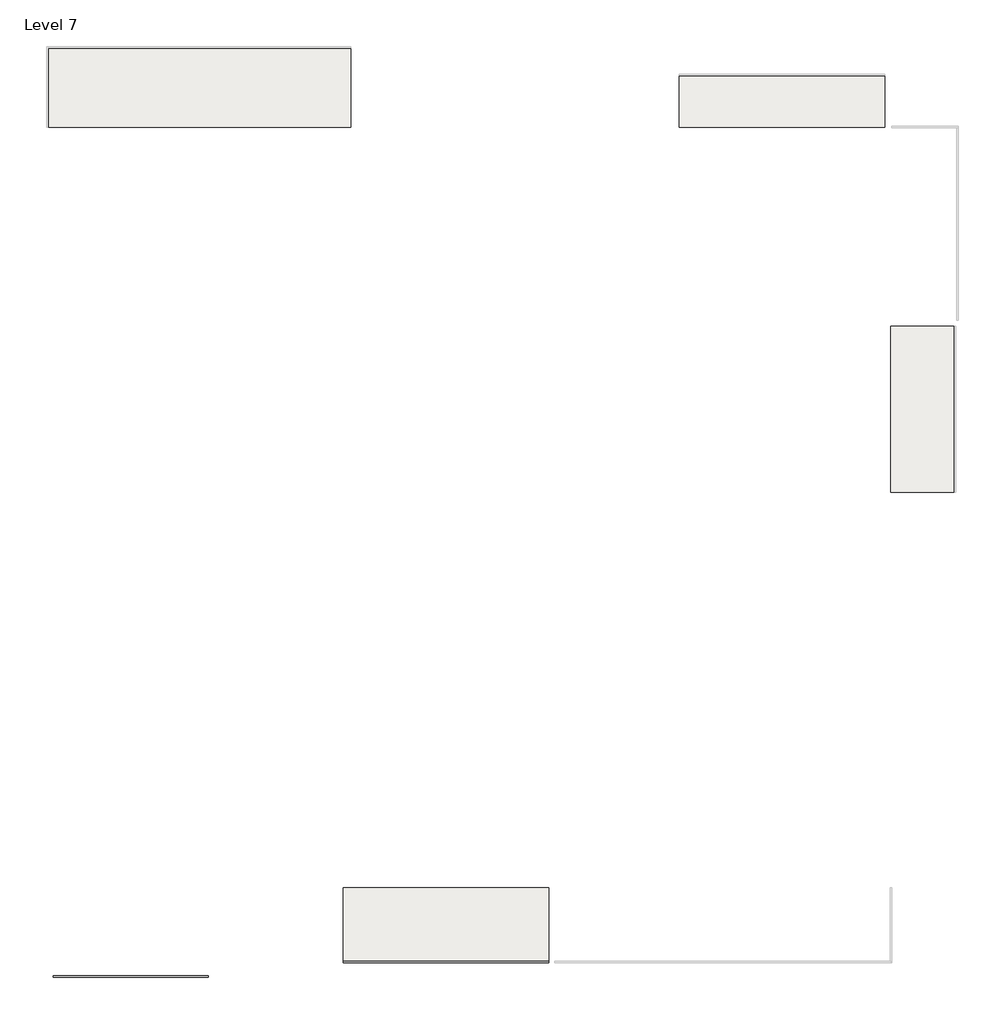
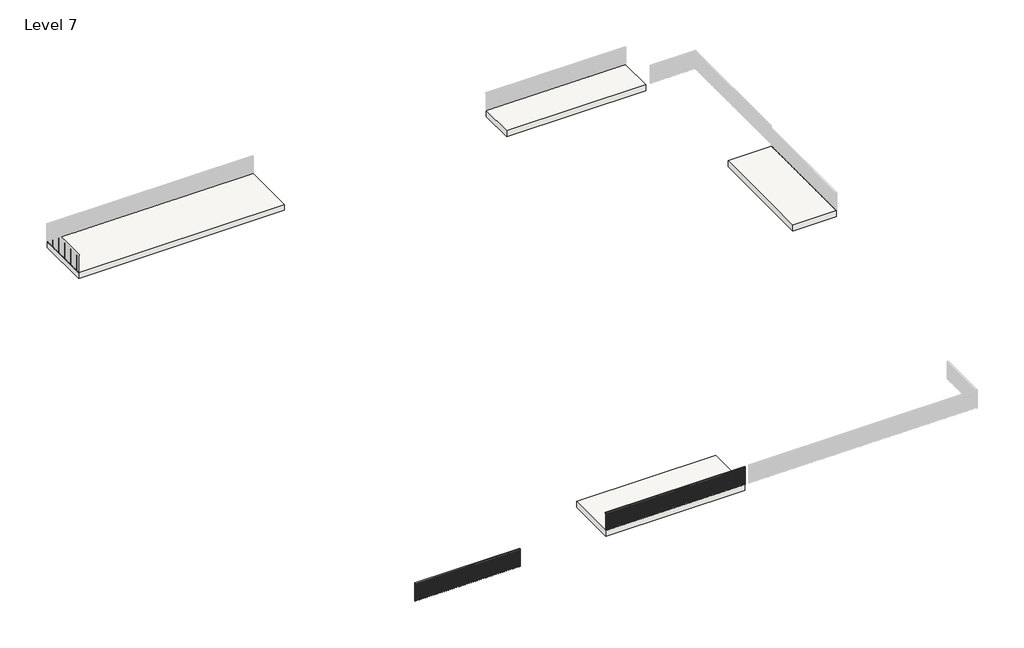
# One storey, part 1 of 5: 4 slabs, 2 railings.
"""IFC4 building model written with IfcOpenShell, lengths in millimetres."""

from ifc_helpers import new_model, si_unit, frame, origin, place, context, project, spatial, polyline, outline, extrude, element, save

model = new_model("IFC4")

# Units and contexts
model_context = context("Model", 3, world=origin())
ifc_project = project(units=[si_unit("LENGTHUNIT", "METRE", prefix="MILLI")], contexts=[model_context])

# Site, building, storey
site = spatial("IfcSite", under=ifc_project)
building = spatial("IfcBuilding", under=site)
storey = spatial("IfcBuildingStorey", under=building, Name="Level 7", Elevation=6400.8)

# Railings
placement = place(None, origin())
element("IfcRailing", 1, ObjectType="Handrail - Rectangular", at=placement, inside=storey, context=model_context, shape_type="SweptSolid", body=[
    extrude(outline(polyline([(-13630.2638778, -13399.9762475), (-13630.2638778, -13349.1762475), (-8499.4638778, -13349.1762475), (-8499.4638778, -13399.9762475), (-13630.2638778, -13399.9762475)])), frame((0.0, 0.0, 7264.4), z_axis=(0.0, 0.0, 1.0), x_axis=(1.0, 0.0, 0.0)), (0.0, 0.0, 1.0), 50.8),
    extrude(outline(polyline([(-8559.7888778, -13384.1012475), (-8559.7888778, -13365.0512475), (-8540.7388778, -13365.0512475), (-8540.7388778, -13384.1012475), (-8559.7888778, -13384.1012475)])), frame((0.0, 0.0, 6400.8), z_axis=(0.0, 0.0, 1.0), x_axis=(1.0, 0.0, 0.0)), (0.0, 0.0, 1.0), 863.6),
    extrude(outline(polyline([(-8661.3888778, -13384.1012475), (-8661.3888778, -13365.0512475), (-8642.3388778, -13365.0512475), (-8642.3388778, -13384.1012475), (-8661.3888778, -13384.1012475)])), frame((0.0, 0.0, 6400.8), z_axis=(0.0, 0.0, 1.0), x_axis=(1.0, 0.0, 0.0)), (0.0, 0.0, 1.0), 863.6),
    extrude(outline(polyline([(-8762.9888778, -13384.1012475), (-8762.9888778, -13365.0512475), (-8743.9388778, -13365.0512475), (-8743.9388778, -13384.1012475), (-8762.9888778, -13384.1012475)])), frame((0.0, 0.0, 6400.8), z_axis=(0.0, 0.0, 1.0), x_axis=(1.0, 0.0, 0.0)), (0.0, 0.0, 1.0), 863.6),
    extrude(outline(polyline([(-8864.5888778, -13384.1012475), (-8864.5888778, -13365.0512475), (-8845.5388778, -13365.0512475), (-8845.5388778, -13384.1012475), (-8864.5888778, -13384.1012475)])), frame((0.0, 0.0, 6400.8), z_axis=(0.0, 0.0, 1.0), x_axis=(1.0, 0.0, 0.0)), (0.0, 0.0, 1.0), 863.6),
    extrude(outline(polyline([(-8966.1888778, -13384.1012475), (-8966.1888778, -13365.0512475), (-8947.1388778, -13365.0512475), (-8947.1388778, -13384.1012475), (-8966.1888778, -13384.1012475)])), frame((0.0, 0.0, 6400.8), z_axis=(0.0, 0.0, 1.0), x_axis=(1.0, 0.0, 0.0)), (0.0, 0.0, 1.0), 863.6),
    extrude(outline(polyline([(-9067.7888778, -13384.1012475), (-9067.7888778, -13365.0512475), (-9048.7388778, -13365.0512475), (-9048.7388778, -13384.1012475), (-9067.7888778, -13384.1012475)])), frame((0.0, 0.0, 6400.8), z_axis=(0.0, 0.0, 1.0), x_axis=(1.0, 0.0, 0.0)), (0.0, 0.0, 1.0), 863.6),
    extrude(outline(polyline([(-9169.3888778, -13384.1012475), (-9169.3888778, -13365.0512475), (-9150.3388778, -13365.0512475), (-9150.3388778, -13384.1012475), (-9169.3888778, -13384.1012475)])), frame((0.0, 0.0, 6400.8), z_axis=(0.0, 0.0, 1.0), x_axis=(1.0, 0.0, 0.0)), (0.0, 0.0, 1.0), 863.6),
    extrude(outline(polyline([(-9270.9888778, -13384.1012475), (-9270.9888778, -13365.0512475), (-9251.9388778, -13365.0512475), (-9251.9388778, -13384.1012475), (-9270.9888778, -13384.1012475)])), frame((0.0, 0.0, 6400.8), z_axis=(0.0, 0.0, 1.0), x_axis=(1.0, 0.0, 0.0)), (0.0, 0.0, 1.0), 863.6),
    extrude(outline(polyline([(-9372.5888778, -13384.1012475), (-9372.5888778, -13365.0512475), (-9353.5388778, -13365.0512475), (-9353.5388778, -13384.1012475), (-9372.5888778, -13384.1012475)])), frame((0.0, 0.0, 6400.8), z_axis=(0.0, 0.0, 1.0), x_axis=(1.0, 0.0, 0.0)), (0.0, 0.0, 1.0), 863.6),
    extrude(outline(polyline([(-9474.1888778, -13384.1012475), (-9474.1888778, -13365.0512475), (-9455.1388778, -13365.0512475), (-9455.1388778, -13384.1012475), (-9474.1888778, -13384.1012475)])), frame((0.0, 0.0, 6400.8), z_axis=(0.0, 0.0, 1.0), x_axis=(1.0, 0.0, 0.0)), (0.0, 0.0, 1.0), 863.6),
    extrude(outline(polyline([(-9575.7888778, -13384.1012475), (-9575.7888778, -13365.0512475), (-9556.7388778, -13365.0512475), (-9556.7388778, -13384.1012475), (-9575.7888778, -13384.1012475)])), frame((0.0, 0.0, 6400.8), z_axis=(0.0, 0.0, 1.0), x_axis=(1.0, 0.0, 0.0)), (0.0, 0.0, 1.0), 863.6),
    extrude(outline(polyline([(-9677.3888778, -13384.1012475), (-9677.3888778, -13365.0512475), (-9658.3388778, -13365.0512475), (-9658.3388778, -13384.1012475), (-9677.3888778, -13384.1012475)])), frame((0.0, 0.0, 6400.8), z_axis=(0.0, 0.0, 1.0), x_axis=(1.0, 0.0, 0.0)), (0.0, 0.0, 1.0), 863.6),
    extrude(outline(polyline([(-9778.9888778, -13384.1012475), (-9778.9888778, -13365.0512475), (-9759.9388778, -13365.0512475), (-9759.9388778, -13384.1012475), (-9778.9888778, -13384.1012475)])), frame((0.0, 0.0, 6400.8), z_axis=(0.0, 0.0, 1.0), x_axis=(1.0, 0.0, 0.0)), (0.0, 0.0, 1.0), 863.6),
    extrude(outline(polyline([(-9880.5888778, -13384.1012475), (-9880.5888778, -13365.0512475), (-9861.5388778, -13365.0512475), (-9861.5388778, -13384.1012475), (-9880.5888778, -13384.1012475)])), frame((0.0, 0.0, 6400.8), z_axis=(0.0, 0.0, 1.0), x_axis=(1.0, 0.0, 0.0)), (0.0, 0.0, 1.0), 863.6),
    extrude(outline(polyline([(-9982.1888778, -13384.1012475), (-9982.1888778, -13365.0512475), (-9963.1388778, -13365.0512475), (-9963.1388778, -13384.1012475), (-9982.1888778, -13384.1012475)])), frame((0.0, 0.0, 6400.8), z_axis=(0.0, 0.0, 1.0), x_axis=(1.0, 0.0, 0.0)), (0.0, 0.0, 1.0), 863.6),
    extrude(outline(polyline([(-10083.7888778, -13384.1012475), (-10083.7888778, -13365.0512475), (-10064.7388778, -13365.0512475), (-10064.7388778, -13384.1012475), (-10083.7888778, -13384.1012475)])), frame((0.0, 0.0, 6400.8), z_axis=(0.0, 0.0, 1.0), x_axis=(1.0, 0.0, 0.0)), (0.0, 0.0, 1.0), 863.6),
    extrude(outline(polyline([(-10185.3888778, -13384.1012475), (-10185.3888778, -13365.0512475), (-10166.3388778, -13365.0512475), (-10166.3388778, -13384.1012475), (-10185.3888778, -13384.1012475)])), frame((0.0, 0.0, 6400.8), z_axis=(0.0, 0.0, 1.0), x_axis=(1.0, 0.0, 0.0)), (0.0, 0.0, 1.0), 863.6),
    extrude(outline(polyline([(-10286.9888778, -13384.1012475), (-10286.9888778, -13365.0512475), (-10267.9388778, -13365.0512475), (-10267.9388778, -13384.1012475), (-10286.9888778, -13384.1012475)])), frame((0.0, 0.0, 6400.8), z_axis=(0.0, 0.0, 1.0), x_axis=(1.0, 0.0, 0.0)), (0.0, 0.0, 1.0), 863.6),
    extrude(outline(polyline([(-10388.5888778, -13384.1012475), (-10388.5888778, -13365.0512475), (-10369.5388778, -13365.0512475), (-10369.5388778, -13384.1012475), (-10388.5888778, -13384.1012475)])), frame((0.0, 0.0, 6400.8), z_axis=(0.0, 0.0, 1.0), x_axis=(1.0, 0.0, 0.0)), (0.0, 0.0, 1.0), 863.6),
    extrude(outline(polyline([(-10490.1888778, -13384.1012475), (-10490.1888778, -13365.0512475), (-10471.1388778, -13365.0512475), (-10471.1388778, -13384.1012475), (-10490.1888778, -13384.1012475)])), frame((0.0, 0.0, 6400.8), z_axis=(0.0, 0.0, 1.0), x_axis=(1.0, 0.0, 0.0)), (0.0, 0.0, 1.0), 863.6),
    extrude(outline(polyline([(-10591.7888778, -13384.1012475), (-10591.7888778, -13365.0512475), (-10572.7388778, -13365.0512475), (-10572.7388778, -13384.1012475), (-10591.7888778, -13384.1012475)])), frame((0.0, 0.0, 6400.8), z_axis=(0.0, 0.0, 1.0), x_axis=(1.0, 0.0, 0.0)), (0.0, 0.0, 1.0), 863.6),
    extrude(outline(polyline([(-10693.3888778, -13384.1012475), (-10693.3888778, -13365.0512475), (-10674.3388778, -13365.0512475), (-10674.3388778, -13384.1012475), (-10693.3888778, -13384.1012475)])), frame((0.0, 0.0, 6400.8), z_axis=(0.0, 0.0, 1.0), x_axis=(1.0, 0.0, 0.0)), (0.0, 0.0, 1.0), 863.6),
    extrude(outline(polyline([(-10794.9888778, -13384.1012475), (-10794.9888778, -13365.0512475), (-10775.9388778, -13365.0512475), (-10775.9388778, -13384.1012475), (-10794.9888778, -13384.1012475)])), frame((0.0, 0.0, 6400.8), z_axis=(0.0, 0.0, 1.0), x_axis=(1.0, 0.0, 0.0)), (0.0, 0.0, 1.0), 863.6),
    extrude(outline(polyline([(-10896.5888778, -13384.1012475), (-10896.5888778, -13365.0512475), (-10877.5388778, -13365.0512475), (-10877.5388778, -13384.1012475), (-10896.5888778, -13384.1012475)])), frame((0.0, 0.0, 6400.8), z_axis=(0.0, 0.0, 1.0), x_axis=(1.0, 0.0, 0.0)), (0.0, 0.0, 1.0), 863.6),
    extrude(outline(polyline([(-10998.1888778, -13384.1012475), (-10998.1888778, -13365.0512475), (-10979.1388778, -13365.0512475), (-10979.1388778, -13384.1012475), (-10998.1888778, -13384.1012475)])), frame((0.0, 0.0, 6400.8), z_axis=(0.0, 0.0, 1.0), x_axis=(1.0, 0.0, 0.0)), (0.0, 0.0, 1.0), 863.6),
    extrude(outline(polyline([(-11099.7888778, -13384.1012475), (-11099.7888778, -13365.0512475), (-11080.7388778, -13365.0512475), (-11080.7388778, -13384.1012475), (-11099.7888778, -13384.1012475)])), frame((0.0, 0.0, 6400.8), z_axis=(0.0, 0.0, 1.0), x_axis=(1.0, 0.0, 0.0)), (0.0, 0.0, 1.0), 863.6),
    extrude(outline(polyline([(-11201.3888778, -13384.1012475), (-11201.3888778, -13365.0512475), (-11182.3388778, -13365.0512475), (-11182.3388778, -13384.1012475), (-11201.3888778, -13384.1012475)])), frame((0.0, 0.0, 6400.8), z_axis=(0.0, 0.0, 1.0), x_axis=(1.0, 0.0, 0.0)), (0.0, 0.0, 1.0), 863.6),
    extrude(outline(polyline([(-11302.9888778, -13384.1012475), (-11302.9888778, -13365.0512475), (-11283.9388778, -13365.0512475), (-11283.9388778, -13384.1012475), (-11302.9888778, -13384.1012475)])), frame((0.0, 0.0, 6400.8), z_axis=(0.0, 0.0, 1.0), x_axis=(1.0, 0.0, 0.0)), (0.0, 0.0, 1.0), 863.6),
    extrude(outline(polyline([(-11404.5888778, -13384.1012475), (-11404.5888778, -13365.0512475), (-11385.5388778, -13365.0512475), (-11385.5388778, -13384.1012475), (-11404.5888778, -13384.1012475)])), frame((0.0, 0.0, 6400.8), z_axis=(0.0, 0.0, 1.0), x_axis=(1.0, 0.0, 0.0)), (0.0, 0.0, 1.0), 863.6),
    extrude(outline(polyline([(-11506.1888778, -13384.1012475), (-11506.1888778, -13365.0512475), (-11487.1388778, -13365.0512475), (-11487.1388778, -13384.1012475), (-11506.1888778, -13384.1012475)])), frame((0.0, 0.0, 6400.8), z_axis=(0.0, 0.0, 1.0), x_axis=(1.0, 0.0, 0.0)), (0.0, 0.0, 1.0), 863.6),
    extrude(outline(polyline([(-11607.7888778, -13384.1012475), (-11607.7888778, -13365.0512475), (-11588.7388778, -13365.0512475), (-11588.7388778, -13384.1012475), (-11607.7888778, -13384.1012475)])), frame((0.0, 0.0, 6400.8), z_axis=(0.0, 0.0, 1.0), x_axis=(1.0, 0.0, 0.0)), (0.0, 0.0, 1.0), 863.6),
    extrude(outline(polyline([(-11709.3888778, -13384.1012475), (-11709.3888778, -13365.0512475), (-11690.3388778, -13365.0512475), (-11690.3388778, -13384.1012475), (-11709.3888778, -13384.1012475)])), frame((0.0, 0.0, 6400.8), z_axis=(0.0, 0.0, 1.0), x_axis=(1.0, 0.0, 0.0)), (0.0, 0.0, 1.0), 863.6),
    extrude(outline(polyline([(-11810.9888778, -13384.1012475), (-11810.9888778, -13365.0512475), (-11791.9388778, -13365.0512475), (-11791.9388778, -13384.1012475), (-11810.9888778, -13384.1012475)])), frame((0.0, 0.0, 6400.8), z_axis=(0.0, 0.0, 1.0), x_axis=(1.0, 0.0, 0.0)), (0.0, 0.0, 1.0), 863.6),
    extrude(outline(polyline([(-11912.5888778, -13384.1012475), (-11912.5888778, -13365.0512475), (-11893.5388778, -13365.0512475), (-11893.5388778, -13384.1012475), (-11912.5888778, -13384.1012475)])), frame((0.0, 0.0, 6400.8), z_axis=(0.0, 0.0, 1.0), x_axis=(1.0, 0.0, 0.0)), (0.0, 0.0, 1.0), 863.6),
    extrude(outline(polyline([(-12014.1888778, -13384.1012475), (-12014.1888778, -13365.0512475), (-11995.1388778, -13365.0512475), (-11995.1388778, -13384.1012475), (-12014.1888778, -13384.1012475)])), frame((0.0, 0.0, 6400.8), z_axis=(0.0, 0.0, 1.0), x_axis=(1.0, 0.0, 0.0)), (0.0, 0.0, 1.0), 863.6),
    extrude(outline(polyline([(-12115.7888778, -13384.1012475), (-12115.7888778, -13365.0512475), (-12096.7388778, -13365.0512475), (-12096.7388778, -13384.1012475), (-12115.7888778, -13384.1012475)])), frame((0.0, 0.0, 6400.8), z_axis=(0.0, 0.0, 1.0), x_axis=(1.0, 0.0, 0.0)), (0.0, 0.0, 1.0), 863.6),
    extrude(outline(polyline([(-12217.3888778, -13384.1012475), (-12217.3888778, -13365.0512475), (-12198.3388778, -13365.0512475), (-12198.3388778, -13384.1012475), (-12217.3888778, -13384.1012475)])), frame((0.0, 0.0, 6400.8), z_axis=(0.0, 0.0, 1.0), x_axis=(1.0, 0.0, 0.0)), (0.0, 0.0, 1.0), 863.6),
    extrude(outline(polyline([(-12318.9888778, -13384.1012475), (-12318.9888778, -13365.0512475), (-12299.9388778, -13365.0512475), (-12299.9388778, -13384.1012475), (-12318.9888778, -13384.1012475)])), frame((0.0, 0.0, 6400.8), z_axis=(0.0, 0.0, 1.0), x_axis=(1.0, 0.0, 0.0)), (0.0, 0.0, 1.0), 863.6),
    extrude(outline(polyline([(-12420.5888778, -13384.1012475), (-12420.5888778, -13365.0512475), (-12401.5388778, -13365.0512475), (-12401.5388778, -13384.1012475), (-12420.5888778, -13384.1012475)])), frame((0.0, 0.0, 6400.8), z_axis=(0.0, 0.0, 1.0), x_axis=(1.0, 0.0, 0.0)), (0.0, 0.0, 1.0), 863.6),
    extrude(outline(polyline([(-12522.1888778, -13384.1012475), (-12522.1888778, -13365.0512475), (-12503.1388778, -13365.0512475), (-12503.1388778, -13384.1012475), (-12522.1888778, -13384.1012475)])), frame((0.0, 0.0, 6400.8), z_axis=(0.0, 0.0, 1.0), x_axis=(1.0, 0.0, 0.0)), (0.0, 0.0, 1.0), 863.6),
    extrude(outline(polyline([(-12623.7888778, -13384.1012475), (-12623.7888778, -13365.0512475), (-12604.7388778, -13365.0512475), (-12604.7388778, -13384.1012475), (-12623.7888778, -13384.1012475)])), frame((0.0, 0.0, 6400.8), z_axis=(0.0, 0.0, 1.0), x_axis=(1.0, 0.0, 0.0)), (0.0, 0.0, 1.0), 863.6),
    extrude(outline(polyline([(-12725.3888778, -13384.1012475), (-12725.3888778, -13365.0512475), (-12706.3388778, -13365.0512475), (-12706.3388778, -13384.1012475), (-12725.3888778, -13384.1012475)])), frame((0.0, 0.0, 6400.8), z_axis=(0.0, 0.0, 1.0), x_axis=(1.0, 0.0, 0.0)), (0.0, 0.0, 1.0), 863.6),
    extrude(outline(polyline([(-12826.9888778, -13384.1012475), (-12826.9888778, -13365.0512475), (-12807.9388778, -13365.0512475), (-12807.9388778, -13384.1012475), (-12826.9888778, -13384.1012475)])), frame((0.0, 0.0, 6400.8), z_axis=(0.0, 0.0, 1.0), x_axis=(1.0, 0.0, 0.0)), (0.0, 0.0, 1.0), 863.6),
    extrude(outline(polyline([(-12928.5888778, -13384.1012475), (-12928.5888778, -13365.0512475), (-12909.5388778, -13365.0512475), (-12909.5388778, -13384.1012475), (-12928.5888778, -13384.1012475)])), frame((0.0, 0.0, 6400.8), z_axis=(0.0, 0.0, 1.0), x_axis=(1.0, 0.0, 0.0)), (0.0, 0.0, 1.0), 863.6),
    extrude(outline(polyline([(-13030.1888778, -13384.1012475), (-13030.1888778, -13365.0512475), (-13011.1388778, -13365.0512475), (-13011.1388778, -13384.1012475), (-13030.1888778, -13384.1012475)])), frame((0.0, 0.0, 6400.8), z_axis=(0.0, 0.0, 1.0), x_axis=(1.0, 0.0, 0.0)), (0.0, 0.0, 1.0), 863.6),
    extrude(outline(polyline([(-13131.7888778, -13384.1012475), (-13131.7888778, -13365.0512475), (-13112.7388778, -13365.0512475), (-13112.7388778, -13384.1012475), (-13131.7888778, -13384.1012475)])), frame((0.0, 0.0, 6400.8), z_axis=(0.0, 0.0, 1.0), x_axis=(1.0, 0.0, 0.0)), (0.0, 0.0, 1.0), 863.6),
    extrude(outline(polyline([(-13233.3888778, -13384.1012475), (-13233.3888778, -13365.0512475), (-13214.3388778, -13365.0512475), (-13214.3388778, -13384.1012475), (-13233.3888778, -13384.1012475)])), frame((0.0, 0.0, 6400.8), z_axis=(0.0, 0.0, 1.0), x_axis=(1.0, 0.0, 0.0)), (0.0, 0.0, 1.0), 863.6),
    extrude(outline(polyline([(-13334.9888778, -13384.1012475), (-13334.9888778, -13365.0512475), (-13315.9388778, -13365.0512475), (-13315.9388778, -13384.1012475), (-13334.9888778, -13384.1012475)])), frame((0.0, 0.0, 6400.8), z_axis=(0.0, 0.0, 1.0), x_axis=(1.0, 0.0, 0.0)), (0.0, 0.0, 1.0), 863.6),
    extrude(outline(polyline([(-13436.5888778, -13384.1012475), (-13436.5888778, -13365.0512475), (-13417.5388778, -13365.0512475), (-13417.5388778, -13384.1012475), (-13436.5888778, -13384.1012475)])), frame((0.0, 0.0, 6400.8), z_axis=(0.0, 0.0, 1.0), x_axis=(1.0, 0.0, 0.0)), (0.0, 0.0, 1.0), 863.6),
    extrude(outline(polyline([(-13538.1888778, -13384.1012475), (-13538.1888778, -13365.0512475), (-13519.1388778, -13365.0512475), (-13519.1388778, -13384.1012475), (-13538.1888778, -13384.1012475)])), frame((0.0, 0.0, 6400.8), z_axis=(0.0, 0.0, 1.0), x_axis=(1.0, 0.0, 0.0)), (0.0, 0.0, 1.0), 863.6),
    extrude(outline(polyline([(-8518.5138778, -13384.1012475), (-8518.5138778, -13365.0512475), (-8499.4638778, -13365.0512475), (-8499.4638778, -13384.1012475), (-8518.5138778, -13384.1012475)])), frame((0.0, 0.0, 6400.8), z_axis=(0.0, 0.0, 1.0), x_axis=(1.0, 0.0, 0.0)), (0.0, 0.0, 1.0), 863.6),
    extrude(outline(polyline([(-13630.2638778, -13384.1012475), (-13630.2638778, -13365.0512475), (-13611.2138778, -13365.0512475), (-13611.2138778, -13384.1012475), (-13630.2638778, -13384.1012475)])), frame((0.0, 0.0, 6400.8), z_axis=(0.0, 0.0, 1.0), x_axis=(1.0, 0.0, 0.0)), (0.0, 0.0, 1.0), 863.6),
])
element("IfcRailing", 2, ObjectType="Handrail - Rectangular", at=placement, inside=storey, context=model_context, shape_type="SweptSolid", body=[
    extrude(outline(polyline([(-4029.0638778, -12911.7749501), (-4029.0638778, -12860.9749501), (2778.1361222, -12860.9749501), (2778.1361222, -12911.7749501), (-4029.0638778, -12911.7749501)])), frame((0.0, 0.0, 7264.4), z_axis=(0.0, 0.0, 1.0), x_axis=(1.0, 0.0, 0.0)), (0.0, 0.0, 1.0), 50.8),
    extrude(outline(polyline([(2667.0111222, -12895.8999501), (2667.0111222, -12876.8499501), (2686.0611222, -12876.8499501), (2686.0611222, -12895.8999501), (2667.0111222, -12895.8999501)])), frame((0.0, 0.0, 6400.8), z_axis=(0.0, 0.0, 1.0), x_axis=(1.0, 0.0, 0.0)), (0.0, 0.0, 1.0), 863.6),
    extrude(outline(polyline([(2565.4111222, -12895.8999501), (2565.4111222, -12876.8499501), (2584.4611222, -12876.8499501), (2584.4611222, -12895.8999501), (2565.4111222, -12895.8999501)])), frame((0.0, 0.0, 6400.8), z_axis=(0.0, 0.0, 1.0), x_axis=(1.0, 0.0, 0.0)), (0.0, 0.0, 1.0), 863.6),
    extrude(outline(polyline([(2463.8111222, -12895.8999501), (2463.8111222, -12876.8499501), (2482.8611222, -12876.8499501), (2482.8611222, -12895.8999501), (2463.8111222, -12895.8999501)])), frame((0.0, 0.0, 6400.8), z_axis=(0.0, 0.0, 1.0), x_axis=(1.0, 0.0, 0.0)), (0.0, 0.0, 1.0), 863.6),
    extrude(outline(polyline([(2362.2111222, -12895.8999501), (2362.2111222, -12876.8499501), (2381.2611222, -12876.8499501), (2381.2611222, -12895.8999501), (2362.2111222, -12895.8999501)])), frame((0.0, 0.0, 6400.8), z_axis=(0.0, 0.0, 1.0), x_axis=(1.0, 0.0, 0.0)), (0.0, 0.0, 1.0), 863.6),
    extrude(outline(polyline([(2260.6111222, -12895.8999501), (2260.6111222, -12876.8499501), (2279.6611222, -12876.8499501), (2279.6611222, -12895.8999501), (2260.6111222, -12895.8999501)])), frame((0.0, 0.0, 6400.8), z_axis=(0.0, 0.0, 1.0), x_axis=(1.0, 0.0, 0.0)), (0.0, 0.0, 1.0), 863.6),
    extrude(outline(polyline([(2159.0111222, -12895.8999501), (2159.0111222, -12876.8499501), (2178.0611222, -12876.8499501), (2178.0611222, -12895.8999501), (2159.0111222, -12895.8999501)])), frame((0.0, 0.0, 6400.8), z_axis=(0.0, 0.0, 1.0), x_axis=(1.0, 0.0, 0.0)), (0.0, 0.0, 1.0), 863.6),
    extrude(outline(polyline([(2057.4111222, -12895.8999501), (2057.4111222, -12876.8499501), (2076.4611222, -12876.8499501), (2076.4611222, -12895.8999501), (2057.4111222, -12895.8999501)])), frame((0.0, 0.0, 6400.8), z_axis=(0.0, 0.0, 1.0), x_axis=(1.0, 0.0, 0.0)), (0.0, 0.0, 1.0), 863.6),
    extrude(outline(polyline([(1955.8111222, -12895.8999501), (1955.8111222, -12876.8499501), (1974.8611222, -12876.8499501), (1974.8611222, -12895.8999501), (1955.8111222, -12895.8999501)])), frame((0.0, 0.0, 6400.8), z_axis=(0.0, 0.0, 1.0), x_axis=(1.0, 0.0, 0.0)), (0.0, 0.0, 1.0), 863.6),
    extrude(outline(polyline([(1854.2111222, -12895.8999501), (1854.2111222, -12876.8499501), (1873.2611222, -12876.8499501), (1873.2611222, -12895.8999501), (1854.2111222, -12895.8999501)])), frame((0.0, 0.0, 6400.8), z_axis=(0.0, 0.0, 1.0), x_axis=(1.0, 0.0, 0.0)), (0.0, 0.0, 1.0), 863.6),
    extrude(outline(polyline([(1752.6111222, -12895.8999501), (1752.6111222, -12876.8499501), (1771.6611222, -12876.8499501), (1771.6611222, -12895.8999501), (1752.6111222, -12895.8999501)])), frame((0.0, 0.0, 6400.8), z_axis=(0.0, 0.0, 1.0), x_axis=(1.0, 0.0, 0.0)), (0.0, 0.0, 1.0), 863.6),
    extrude(outline(polyline([(1651.0111222, -12895.8999501), (1651.0111222, -12876.8499501), (1670.0611222, -12876.8499501), (1670.0611222, -12895.8999501), (1651.0111222, -12895.8999501)])), frame((0.0, 0.0, 6400.8), z_axis=(0.0, 0.0, 1.0), x_axis=(1.0, 0.0, 0.0)), (0.0, 0.0, 1.0), 863.6),
    extrude(outline(polyline([(1549.4111222, -12895.8999501), (1549.4111222, -12876.8499501), (1568.4611222, -12876.8499501), (1568.4611222, -12895.8999501), (1549.4111222, -12895.8999501)])), frame((0.0, 0.0, 6400.8), z_axis=(0.0, 0.0, 1.0), x_axis=(1.0, 0.0, 0.0)), (0.0, 0.0, 1.0), 863.6),
    extrude(outline(polyline([(1447.8111222, -12895.8999501), (1447.8111222, -12876.8499501), (1466.8611222, -12876.8499501), (1466.8611222, -12895.8999501), (1447.8111222, -12895.8999501)])), frame((0.0, 0.0, 6400.8), z_axis=(0.0, 0.0, 1.0), x_axis=(1.0, 0.0, 0.0)), (0.0, 0.0, 1.0), 863.6),
    extrude(outline(polyline([(1346.2111222, -12895.8999501), (1346.2111222, -12876.8499501), (1365.2611222, -12876.8499501), (1365.2611222, -12895.8999501), (1346.2111222, -12895.8999501)])), frame((0.0, 0.0, 6400.8), z_axis=(0.0, 0.0, 1.0), x_axis=(1.0, 0.0, 0.0)), (0.0, 0.0, 1.0), 863.6),
    extrude(outline(polyline([(1244.6111222, -12895.8999501), (1244.6111222, -12876.8499501), (1263.6611222, -12876.8499501), (1263.6611222, -12895.8999501), (1244.6111222, -12895.8999501)])), frame((0.0, 0.0, 6400.8), z_axis=(0.0, 0.0, 1.0), x_axis=(1.0, 0.0, 0.0)), (0.0, 0.0, 1.0), 863.6),
    extrude(outline(polyline([(1143.0111222, -12895.8999501), (1143.0111222, -12876.8499501), (1162.0611222, -12876.8499501), (1162.0611222, -12895.8999501), (1143.0111222, -12895.8999501)])), frame((0.0, 0.0, 6400.8), z_axis=(0.0, 0.0, 1.0), x_axis=(1.0, 0.0, 0.0)), (0.0, 0.0, 1.0), 863.6),
    extrude(outline(polyline([(1041.4111222, -12895.8999501), (1041.4111222, -12876.8499501), (1060.4611222, -12876.8499501), (1060.4611222, -12895.8999501), (1041.4111222, -12895.8999501)])), frame((0.0, 0.0, 6400.8), z_axis=(0.0, 0.0, 1.0), x_axis=(1.0, 0.0, 0.0)), (0.0, 0.0, 1.0), 863.6),
    extrude(outline(polyline([(939.8111222, -12895.8999501), (939.8111222, -12876.8499501), (958.8611222, -12876.8499501), (958.8611222, -12895.8999501), (939.8111222, -12895.8999501)])), frame((0.0, 0.0, 6400.8), z_axis=(0.0, 0.0, 1.0), x_axis=(1.0, 0.0, 0.0)), (0.0, 0.0, 1.0), 863.6),
    extrude(outline(polyline([(838.2111222, -12895.8999501), (838.2111222, -12876.8499501), (857.2611222, -12876.8499501), (857.2611222, -12895.8999501), (838.2111222, -12895.8999501)])), frame((0.0, 0.0, 6400.8), z_axis=(0.0, 0.0, 1.0), x_axis=(1.0, 0.0, 0.0)), (0.0, 0.0, 1.0), 863.6),
    extrude(outline(polyline([(736.6111222, -12895.8999501), (736.6111222, -12876.8499501), (755.6611222, -12876.8499501), (755.6611222, -12895.8999501), (736.6111222, -12895.8999501)])), frame((0.0, 0.0, 6400.8), z_axis=(0.0, 0.0, 1.0), x_axis=(1.0, 0.0, 0.0)), (0.0, 0.0, 1.0), 863.6),
    extrude(outline(polyline([(635.0111222, -12895.8999501), (635.0111222, -12876.8499501), (654.0611222, -12876.8499501), (654.0611222, -12895.8999501), (635.0111222, -12895.8999501)])), frame((0.0, 0.0, 6400.8), z_axis=(0.0, 0.0, 1.0), x_axis=(1.0, 0.0, 0.0)), (0.0, 0.0, 1.0), 863.6),
    extrude(outline(polyline([(533.4111222, -12895.8999501), (533.4111222, -12876.8499501), (552.4611222, -12876.8499501), (552.4611222, -12895.8999501), (533.4111222, -12895.8999501)])), frame((0.0, 0.0, 6400.8), z_axis=(0.0, 0.0, 1.0), x_axis=(1.0, 0.0, 0.0)), (0.0, 0.0, 1.0), 863.6),
    extrude(outline(polyline([(431.8111222, -12895.8999501), (431.8111222, -12876.8499501), (450.8611222, -12876.8499501), (450.8611222, -12895.8999501), (431.8111222, -12895.8999501)])), frame((0.0, 0.0, 6400.8), z_axis=(0.0, 0.0, 1.0), x_axis=(1.0, 0.0, 0.0)), (0.0, 0.0, 1.0), 863.6),
    extrude(outline(polyline([(330.2111222, -12895.8999501), (330.2111222, -12876.8499501), (349.2611222, -12876.8499501), (349.2611222, -12895.8999501), (330.2111222, -12895.8999501)])), frame((0.0, 0.0, 6400.8), z_axis=(0.0, 0.0, 1.0), x_axis=(1.0, 0.0, 0.0)), (0.0, 0.0, 1.0), 863.6),
    extrude(outline(polyline([(228.6111222, -12895.8999501), (228.6111222, -12876.8499501), (247.6611222, -12876.8499501), (247.6611222, -12895.8999501), (228.6111222, -12895.8999501)])), frame((0.0, 0.0, 6400.8), z_axis=(0.0, 0.0, 1.0), x_axis=(1.0, 0.0, 0.0)), (0.0, 0.0, 1.0), 863.6),
    extrude(outline(polyline([(127.0111222, -12895.8999501), (127.0111222, -12876.8499501), (146.0611222, -12876.8499501), (146.0611222, -12895.8999501), (127.0111222, -12895.8999501)])), frame((0.0, 0.0, 6400.8), z_axis=(0.0, 0.0, 1.0), x_axis=(1.0, 0.0, 0.0)), (0.0, 0.0, 1.0), 863.6),
    extrude(outline(polyline([(25.4111222, -12895.8999501), (25.4111222, -12876.8499501), (44.4611222, -12876.8499501), (44.4611222, -12895.8999501), (25.4111222, -12895.8999501)])), frame((0.0, 0.0, 6400.8), z_axis=(0.0, 0.0, 1.0), x_axis=(1.0, 0.0, 0.0)), (0.0, 0.0, 1.0), 863.6),
    extrude(outline(polyline([(-76.1888778, -12895.8999501), (-76.1888778, -12876.8499501), (-57.1388778, -12876.8499501), (-57.1388778, -12895.8999501), (-76.1888778, -12895.8999501)])), frame((0.0, 0.0, 6400.8), z_axis=(0.0, 0.0, 1.0), x_axis=(1.0, 0.0, 0.0)), (0.0, 0.0, 1.0), 863.6),
    extrude(outline(polyline([(-177.7888778, -12895.8999501), (-177.7888778, -12876.8499501), (-158.7388778, -12876.8499501), (-158.7388778, -12895.8999501), (-177.7888778, -12895.8999501)])), frame((0.0, 0.0, 6400.8), z_axis=(0.0, 0.0, 1.0), x_axis=(1.0, 0.0, 0.0)), (0.0, 0.0, 1.0), 863.6),
    extrude(outline(polyline([(-279.3888778, -12895.8999501), (-279.3888778, -12876.8499501), (-260.3388778, -12876.8499501), (-260.3388778, -12895.8999501), (-279.3888778, -12895.8999501)])), frame((0.0, 0.0, 6400.8), z_axis=(0.0, 0.0, 1.0), x_axis=(1.0, 0.0, 0.0)), (0.0, 0.0, 1.0), 863.6),
    extrude(outline(polyline([(-380.9888778, -12895.8999501), (-380.9888778, -12876.8499501), (-361.9388778, -12876.8499501), (-361.9388778, -12895.8999501), (-380.9888778, -12895.8999501)])), frame((0.0, 0.0, 6400.8), z_axis=(0.0, 0.0, 1.0), x_axis=(1.0, 0.0, 0.0)), (0.0, 0.0, 1.0), 863.6),
    extrude(outline(polyline([(-482.5888778, -12895.8999501), (-482.5888778, -12876.8499501), (-463.5388778, -12876.8499501), (-463.5388778, -12895.8999501), (-482.5888778, -12895.8999501)])), frame((0.0, 0.0, 6400.8), z_axis=(0.0, 0.0, 1.0), x_axis=(1.0, 0.0, 0.0)), (0.0, 0.0, 1.0), 863.6),
    extrude(outline(polyline([(-584.1888778, -12895.8999501), (-584.1888778, -12876.8499501), (-565.1388778, -12876.8499501), (-565.1388778, -12895.8999501), (-584.1888778, -12895.8999501)])), frame((0.0, 0.0, 6400.8), z_axis=(0.0, 0.0, 1.0), x_axis=(1.0, 0.0, 0.0)), (0.0, 0.0, 1.0), 863.6),
    extrude(outline(polyline([(-685.7888778, -12895.8999501), (-685.7888778, -12876.8499501), (-666.7388778, -12876.8499501), (-666.7388778, -12895.8999501), (-685.7888778, -12895.8999501)])), frame((0.0, 0.0, 6400.8), z_axis=(0.0, 0.0, 1.0), x_axis=(1.0, 0.0, 0.0)), (0.0, 0.0, 1.0), 863.6),
    extrude(outline(polyline([(-787.3888778, -12895.8999501), (-787.3888778, -12876.8499501), (-768.3388778, -12876.8499501), (-768.3388778, -12895.8999501), (-787.3888778, -12895.8999501)])), frame((0.0, 0.0, 6400.8), z_axis=(0.0, 0.0, 1.0), x_axis=(1.0, 0.0, 0.0)), (0.0, 0.0, 1.0), 863.6),
    extrude(outline(polyline([(-888.9888778, -12895.8999501), (-888.9888778, -12876.8499501), (-869.9388778, -12876.8499501), (-869.9388778, -12895.8999501), (-888.9888778, -12895.8999501)])), frame((0.0, 0.0, 6400.8), z_axis=(0.0, 0.0, 1.0), x_axis=(1.0, 0.0, 0.0)), (0.0, 0.0, 1.0), 863.6),
    extrude(outline(polyline([(-990.5888778, -12895.8999501), (-990.5888778, -12876.8499501), (-971.5388778, -12876.8499501), (-971.5388778, -12895.8999501), (-990.5888778, -12895.8999501)])), frame((0.0, 0.0, 6400.8), z_axis=(0.0, 0.0, 1.0), x_axis=(1.0, 0.0, 0.0)), (0.0, 0.0, 1.0), 863.6),
    extrude(outline(polyline([(-1092.1888778, -12895.8999501), (-1092.1888778, -12876.8499501), (-1073.1388778, -12876.8499501), (-1073.1388778, -12895.8999501), (-1092.1888778, -12895.8999501)])), frame((0.0, 0.0, 6400.8), z_axis=(0.0, 0.0, 1.0), x_axis=(1.0, 0.0, 0.0)), (0.0, 0.0, 1.0), 863.6),
    extrude(outline(polyline([(-1193.7888778, -12895.8999501), (-1193.7888778, -12876.8499501), (-1174.7388778, -12876.8499501), (-1174.7388778, -12895.8999501), (-1193.7888778, -12895.8999501)])), frame((0.0, 0.0, 6400.8), z_axis=(0.0, 0.0, 1.0), x_axis=(1.0, 0.0, 0.0)), (0.0, 0.0, 1.0), 863.6),
    extrude(outline(polyline([(-1295.3888778, -12895.8999501), (-1295.3888778, -12876.8499501), (-1276.3388778, -12876.8499501), (-1276.3388778, -12895.8999501), (-1295.3888778, -12895.8999501)])), frame((0.0, 0.0, 6400.8), z_axis=(0.0, 0.0, 1.0), x_axis=(1.0, 0.0, 0.0)), (0.0, 0.0, 1.0), 863.6),
    extrude(outline(polyline([(-1396.9888778, -12895.8999501), (-1396.9888778, -12876.8499501), (-1377.9388778, -12876.8499501), (-1377.9388778, -12895.8999501), (-1396.9888778, -12895.8999501)])), frame((0.0, 0.0, 6400.8), z_axis=(0.0, 0.0, 1.0), x_axis=(1.0, 0.0, 0.0)), (0.0, 0.0, 1.0), 863.6),
    extrude(outline(polyline([(-1498.5888778, -12895.8999501), (-1498.5888778, -12876.8499501), (-1479.5388778, -12876.8499501), (-1479.5388778, -12895.8999501), (-1498.5888778, -12895.8999501)])), frame((0.0, 0.0, 6400.8), z_axis=(0.0, 0.0, 1.0), x_axis=(1.0, 0.0, 0.0)), (0.0, 0.0, 1.0), 863.6),
    extrude(outline(polyline([(-1600.1888778, -12895.8999501), (-1600.1888778, -12876.8499501), (-1581.1388778, -12876.8499501), (-1581.1388778, -12895.8999501), (-1600.1888778, -12895.8999501)])), frame((0.0, 0.0, 6400.8), z_axis=(0.0, 0.0, 1.0), x_axis=(1.0, 0.0, 0.0)), (0.0, 0.0, 1.0), 863.6),
    extrude(outline(polyline([(-1701.7888778, -12895.8999501), (-1701.7888778, -12876.8499501), (-1682.7388778, -12876.8499501), (-1682.7388778, -12895.8999501), (-1701.7888778, -12895.8999501)])), frame((0.0, 0.0, 6400.8), z_axis=(0.0, 0.0, 1.0), x_axis=(1.0, 0.0, 0.0)), (0.0, 0.0, 1.0), 863.6),
    extrude(outline(polyline([(-1803.3888778, -12895.8999501), (-1803.3888778, -12876.8499501), (-1784.3388778, -12876.8499501), (-1784.3388778, -12895.8999501), (-1803.3888778, -12895.8999501)])), frame((0.0, 0.0, 6400.8), z_axis=(0.0, 0.0, 1.0), x_axis=(1.0, 0.0, 0.0)), (0.0, 0.0, 1.0), 863.6),
    extrude(outline(polyline([(-1904.9888778, -12895.8999501), (-1904.9888778, -12876.8499501), (-1885.9388778, -12876.8499501), (-1885.9388778, -12895.8999501), (-1904.9888778, -12895.8999501)])), frame((0.0, 0.0, 6400.8), z_axis=(0.0, 0.0, 1.0), x_axis=(1.0, 0.0, 0.0)), (0.0, 0.0, 1.0), 863.6),
    extrude(outline(polyline([(-2006.5888778, -12895.8999501), (-2006.5888778, -12876.8499501), (-1987.5388778, -12876.8499501), (-1987.5388778, -12895.8999501), (-2006.5888778, -12895.8999501)])), frame((0.0, 0.0, 6400.8), z_axis=(0.0, 0.0, 1.0), x_axis=(1.0, 0.0, 0.0)), (0.0, 0.0, 1.0), 863.6),
    extrude(outline(polyline([(-2108.1888778, -12895.8999501), (-2108.1888778, -12876.8499501), (-2089.1388778, -12876.8499501), (-2089.1388778, -12895.8999501), (-2108.1888778, -12895.8999501)])), frame((0.0, 0.0, 6400.8), z_axis=(0.0, 0.0, 1.0), x_axis=(1.0, 0.0, 0.0)), (0.0, 0.0, 1.0), 863.6),
    extrude(outline(polyline([(-2209.7888778, -12895.8999501), (-2209.7888778, -12876.8499501), (-2190.7388778, -12876.8499501), (-2190.7388778, -12895.8999501), (-2209.7888778, -12895.8999501)])), frame((0.0, 0.0, 6400.8), z_axis=(0.0, 0.0, 1.0), x_axis=(1.0, 0.0, 0.0)), (0.0, 0.0, 1.0), 863.6),
    extrude(outline(polyline([(-2311.3888778, -12895.8999501), (-2311.3888778, -12876.8499501), (-2292.3388778, -12876.8499501), (-2292.3388778, -12895.8999501), (-2311.3888778, -12895.8999501)])), frame((0.0, 0.0, 6400.8), z_axis=(0.0, 0.0, 1.0), x_axis=(1.0, 0.0, 0.0)), (0.0, 0.0, 1.0), 863.6),
    extrude(outline(polyline([(-2412.9888778, -12895.8999501), (-2412.9888778, -12876.8499501), (-2393.9388778, -12876.8499501), (-2393.9388778, -12895.8999501), (-2412.9888778, -12895.8999501)])), frame((0.0, 0.0, 6400.8), z_axis=(0.0, 0.0, 1.0), x_axis=(1.0, 0.0, 0.0)), (0.0, 0.0, 1.0), 863.6),
    extrude(outline(polyline([(-2514.5888778, -12895.8999501), (-2514.5888778, -12876.8499501), (-2495.5388778, -12876.8499501), (-2495.5388778, -12895.8999501), (-2514.5888778, -12895.8999501)])), frame((0.0, 0.0, 6400.8), z_axis=(0.0, 0.0, 1.0), x_axis=(1.0, 0.0, 0.0)), (0.0, 0.0, 1.0), 863.6),
    extrude(outline(polyline([(-2616.1888778, -12895.8999501), (-2616.1888778, -12876.8499501), (-2597.1388778, -12876.8499501), (-2597.1388778, -12895.8999501), (-2616.1888778, -12895.8999501)])), frame((0.0, 0.0, 6400.8), z_axis=(0.0, 0.0, 1.0), x_axis=(1.0, 0.0, 0.0)), (0.0, 0.0, 1.0), 863.6),
    extrude(outline(polyline([(-2717.7888778, -12895.8999501), (-2717.7888778, -12876.8499501), (-2698.7388778, -12876.8499501), (-2698.7388778, -12895.8999501), (-2717.7888778, -12895.8999501)])), frame((0.0, 0.0, 6400.8), z_axis=(0.0, 0.0, 1.0), x_axis=(1.0, 0.0, 0.0)), (0.0, 0.0, 1.0), 863.6),
    extrude(outline(polyline([(-2819.3888778, -12895.8999501), (-2819.3888778, -12876.8499501), (-2800.3388778, -12876.8499501), (-2800.3388778, -12895.8999501), (-2819.3888778, -12895.8999501)])), frame((0.0, 0.0, 6400.8), z_axis=(0.0, 0.0, 1.0), x_axis=(1.0, 0.0, 0.0)), (0.0, 0.0, 1.0), 863.6),
    extrude(outline(polyline([(-2920.9888778, -12895.8999501), (-2920.9888778, -12876.8499501), (-2901.9388778, -12876.8499501), (-2901.9388778, -12895.8999501), (-2920.9888778, -12895.8999501)])), frame((0.0, 0.0, 6400.8), z_axis=(0.0, 0.0, 1.0), x_axis=(1.0, 0.0, 0.0)), (0.0, 0.0, 1.0), 863.6),
    extrude(outline(polyline([(-3022.5888778, -12895.8999501), (-3022.5888778, -12876.8499501), (-3003.5388778, -12876.8499501), (-3003.5388778, -12895.8999501), (-3022.5888778, -12895.8999501)])), frame((0.0, 0.0, 6400.8), z_axis=(0.0, 0.0, 1.0), x_axis=(1.0, 0.0, 0.0)), (0.0, 0.0, 1.0), 863.6),
    extrude(outline(polyline([(-3124.1888778, -12895.8999501), (-3124.1888778, -12876.8499501), (-3105.1388778, -12876.8499501), (-3105.1388778, -12895.8999501), (-3124.1888778, -12895.8999501)])), frame((0.0, 0.0, 6400.8), z_axis=(0.0, 0.0, 1.0), x_axis=(1.0, 0.0, 0.0)), (0.0, 0.0, 1.0), 863.6),
    extrude(outline(polyline([(-3225.7888778, -12895.8999501), (-3225.7888778, -12876.8499501), (-3206.7388778, -12876.8499501), (-3206.7388778, -12895.8999501), (-3225.7888778, -12895.8999501)])), frame((0.0, 0.0, 6400.8), z_axis=(0.0, 0.0, 1.0), x_axis=(1.0, 0.0, 0.0)), (0.0, 0.0, 1.0), 863.6),
    extrude(outline(polyline([(-3327.3888778, -12895.8999501), (-3327.3888778, -12876.8499501), (-3308.3388778, -12876.8499501), (-3308.3388778, -12895.8999501), (-3327.3888778, -12895.8999501)])), frame((0.0, 0.0, 6400.8), z_axis=(0.0, 0.0, 1.0), x_axis=(1.0, 0.0, 0.0)), (0.0, 0.0, 1.0), 863.6),
    extrude(outline(polyline([(-3428.9888778, -12895.8999501), (-3428.9888778, -12876.8499501), (-3409.9388778, -12876.8499501), (-3409.9388778, -12895.8999501), (-3428.9888778, -12895.8999501)])), frame((0.0, 0.0, 6400.8), z_axis=(0.0, 0.0, 1.0), x_axis=(1.0, 0.0, 0.0)), (0.0, 0.0, 1.0), 863.6),
    extrude(outline(polyline([(-3530.5888778, -12895.8999501), (-3530.5888778, -12876.8499501), (-3511.5388778, -12876.8499501), (-3511.5388778, -12895.8999501), (-3530.5888778, -12895.8999501)])), frame((0.0, 0.0, 6400.8), z_axis=(0.0, 0.0, 1.0), x_axis=(1.0, 0.0, 0.0)), (0.0, 0.0, 1.0), 863.6),
    extrude(outline(polyline([(-3632.1888778, -12895.8999501), (-3632.1888778, -12876.8499501), (-3613.1388778, -12876.8499501), (-3613.1388778, -12895.8999501), (-3632.1888778, -12895.8999501)])), frame((0.0, 0.0, 6400.8), z_axis=(0.0, 0.0, 1.0), x_axis=(1.0, 0.0, 0.0)), (0.0, 0.0, 1.0), 863.6),
    extrude(outline(polyline([(-3733.7888778, -12895.8999501), (-3733.7888778, -12876.8499501), (-3714.7388778, -12876.8499501), (-3714.7388778, -12895.8999501), (-3733.7888778, -12895.8999501)])), frame((0.0, 0.0, 6400.8), z_axis=(0.0, 0.0, 1.0), x_axis=(1.0, 0.0, 0.0)), (0.0, 0.0, 1.0), 863.6),
    extrude(outline(polyline([(-3835.3888778, -12895.8999501), (-3835.3888778, -12876.8499501), (-3816.3388778, -12876.8499501), (-3816.3388778, -12895.8999501), (-3835.3888778, -12895.8999501)])), frame((0.0, 0.0, 6400.8), z_axis=(0.0, 0.0, 1.0), x_axis=(1.0, 0.0, 0.0)), (0.0, 0.0, 1.0), 863.6),
    extrude(outline(polyline([(-3936.9888778, -12895.8999501), (-3936.9888778, -12876.8499501), (-3917.9388778, -12876.8499501), (-3917.9388778, -12895.8999501), (-3936.9888778, -12895.8999501)])), frame((0.0, 0.0, 6400.8), z_axis=(0.0, 0.0, 1.0), x_axis=(1.0, 0.0, 0.0)), (0.0, 0.0, 1.0), 863.6),
    extrude(outline(polyline([(2759.0861222, -12895.8999501), (2759.0861222, -12876.8499501), (2778.1361222, -12876.8499501), (2778.1361222, -12895.8999501), (2759.0861222, -12895.8999501)])), frame((0.0, 0.0, 6400.8), z_axis=(0.0, 0.0, 1.0), x_axis=(1.0, 0.0, 0.0)), (0.0, 0.0, 1.0), 863.6),
    extrude(outline(polyline([(-4029.0638778, -12895.8999501), (-4029.0638778, -12876.8499501), (-4010.0138778, -12876.8499501), (-4010.0138778, -12895.8999501), (-4029.0638778, -12895.8999501)])), frame((0.0, 0.0, 6400.8), z_axis=(0.0, 0.0, 1.0), x_axis=(1.0, 0.0, 0.0)), (0.0, 0.0, 1.0), 863.6),
])

# Slabs
element("IfcSlab", 3, at=placement, inside=storey, context=model_context, shape_type="SweptSolid", body=[
    extrude(outline(polyline([(-13833.4638778, 14768.6237525), (-13833.4638778, 17410.2237525), (-3775.0638778, 17410.2237525), (-3775.0638778, 14768.6237525), (-13833.4638778, 14768.6237525)])), frame((0.0, 0.0, 6096.0), z_axis=(0.0, 0.0, 1.0), x_axis=(1.0, 0.0, 0.0)), (0.0, 0.0, 1.0), 304.8),
])
element("IfcSlab", 4, ObjectType="Generic - 12\"", at=placement, inside=storey, context=model_context, shape_type="SweptSolid", body=[
    extrude(outline(polyline([(2778.1361222, -10428.1762475), (2778.1361222, -12886.3749501), (-4029.0638778, -12886.3749501), (-4029.0638778, -10428.1762475), (2778.1361222, -10428.1762475)])), frame((0.0, 0.0, 6096.0), z_axis=(0.0, 0.0, 1.0), x_axis=(1.0, 0.0, 0.0)), (0.0, 0.0, 1.0), 304.8),
])
element("IfcSlab", 5, ObjectType="Generic - 12\"", at=placement, inside=storey, context=model_context, shape_type="SweptSolid", body=[
    extrude(outline(polyline([(16240.1361222, 8164.6237525), (16240.1361222, 2678.2237525), (14106.5361222, 2678.2237525), (14106.5361222, 8164.6237525), (16240.1361222, 8164.6237525)])), frame((0.0, 0.0, 6096.0), z_axis=(0.0, 0.0, 1.0), x_axis=(1.0, 0.0, 0.0)), (0.0, 0.0, 1.0), 304.8),
])
element("IfcSlab", 6, ObjectType="Generic - 12\"", at=placement, inside=storey, context=model_context, shape_type="SweptSolid", body=[
    extrude(outline(polyline([(7096.1361222, 14768.6237525), (7096.1361222, 16495.8237525), (13903.3361222, 16495.8237525), (13903.3361222, 14768.6237525), (7096.1361222, 14768.6237525)])), frame((0.0, 0.0, 6096.0), z_axis=(0.0, 0.0, 1.0), x_axis=(1.0, 0.0, 0.0)), (0.0, 0.0, 1.0), 304.8),
])

save(model, "model.ifc")

# Revit data of these elements
# Type "Handrail - Rectangular"
#   Assembly Code = "C2010400"
#   built-in parameter 1008612 = 0.0416667 (stored number, unit not read)
#   built-in parameter 1008611 = 0.0416667 (stored number, unit not read)
#   built-in parameter 1008609 = 0.333333 (stored number, unit not read)
#   built-in parameter 1008604 = 0.166667 (stored number, unit not read)
#   built-in parameter 1008603 = 0.166667 (stored number, unit not read)
#   Railing Height = 3' - 0"
#   built-in parameter 1008630 = 2
#   built-in parameter 1008610 = 2
#   built-in parameter 1008618 = Baluster - Square : 3/4"
# Type
#   Assembly Code = "B1010"
#   Function = 0
#   Layers, outside or top first: 1' - 0" "Tile, Porcelain, 4in" (function 1)
# Type "Generic - 12\""
#   Assembly Code = "B1010"
#   Function = 0
#   Layers, outside or top first: 1' - 0" no material (function 1)
# Elements 1, 2 (IfcRailing, "Handrail - Rectangular")
#   Phase Created = New Construction
# Element 3 (IfcSlab)
#   built-in parameter 1001955 = 3.14159 (stored number, unit not read)
#   Height Offset From Level = 0' - 0"
#   Phase Created = New Construction
#   Materials on its faces: "Tile, Porcelain, 4in"
# Elements 4, 5 (IfcSlab, "Generic - 12\"")
#   Height Offset From Level = 0' - 0"
#   Phase Created = New Construction
#   Materials on its faces: "Default Floor"
# Element 6 (IfcSlab, "Generic - 12\"")
#   built-in parameter 1001955 = 3.14159 (stored number, unit not read)
#   Height Offset From Level = 0' - 0"
#   Phase Created = New Construction
#   Materials on its faces: "Default Floor"
# Materials
#   "Tile, Porcelain, 4in": class "Generic", colour RGB 89 87 158, transparency 0, Description = "Porcelain tile, 4\", white", Cost = 0
#   "Default Floor": colour RGB 128 128 128, transparency 0
